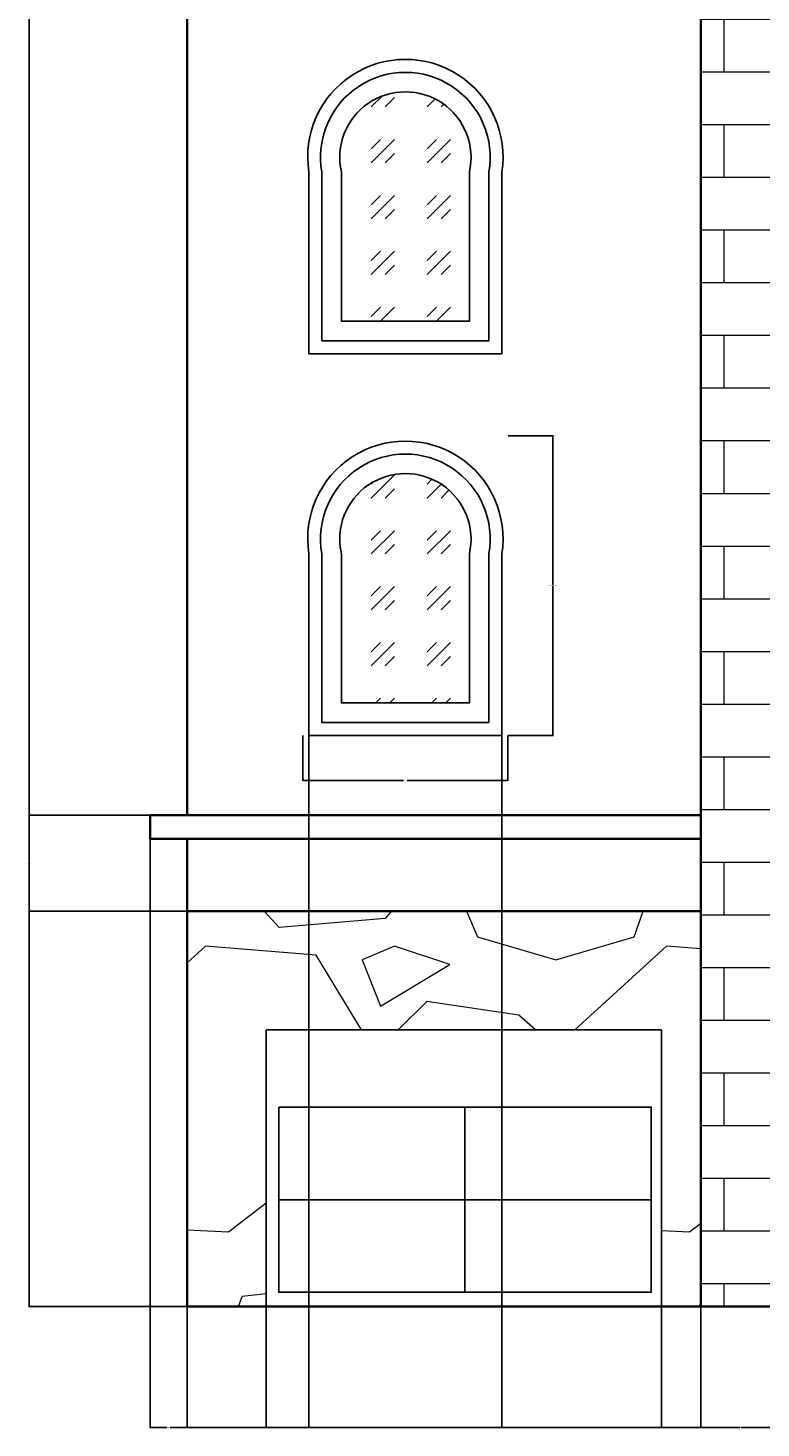
# Model space of a CAD drawing. Units: inches. Extents: x -19 to 556, y -28 to 766.
# Tile 1 of 3: x -19 to 203, y -28 to 397. Entities that reach past the tile are written whole.
import ezdxf

# ---------------------------------------------------------------- set-up
doc = ezdxf.new("R2010")
doc.units = ezdxf.units.IN
doc.header["$MEASUREMENT"] = 0
for name, color, linetype, lineweight in [('A-ANNO-DIMS', 2, 'Continuous', 18), ('A-DOOR', 3, 'Continuous', 25), ('A-ELEV', 7, 'Continuous', 35), ('A-GLAZ', 4, 'Continuous', 25), ('A-GLAZ-PATT', 252, 'Continuous', 13), ('A-WALL-PATT', 8, 'Continuous', 13)]:
    doc.layers.add(name, color=color, linetype=linetype, lineweight=lineweight)
doc.styles.get("Standard").update_dxf_attribs({"font": 'arial.ttf'})
doc.dimstyles.get("Standard").update_dxf_attribs({"dimtxt": 0.18, "dimasz": 0.18, "dimexe": 0.18, "dimexo": 0.0625, "dimgap": 0.09, "dimtad": 0, "dimtih": 1, "dimtoh": 1, "dimdec": 4, "dimzin": 0, "dimdsep": 46, "dimtxsty": 'Standard', "dimcen": 0.09, "dimadec": 0, "dimazin": 0, "dimtfac": 1, "dimtdec": 4, "dimtofl": 0, "dimtmove": 0, "dimatfit": 3, "dimfxl": 1, "dimtolj": 1, "dimtzin": 0, "dimarcsym": 0})

# ---------------------------------------------------------------- blocks, each defined once
blk = doc.blocks.new('WIN-ARCHED')
for points in [[(65.94, 237.64), (65.94, 182.48), (124.55, 182.48), (124.55, 237.64, 1.168317)], [(69.88, 237.64), (69.88, 186.43), (120.6, 186.43), (120.6, 237.64, 1.194508)], [(75.8, 237.64), (75.8, 192.35), (114.68, 192.35), (114.68, 237.64, 1.253731)]]:
    blk.add_lwpolyline(points, format="xyb", close=True)
blk = doc.blocks.new('DOOR-GARAGE')
for p, q in [((113.34, 69.59), (113.34, 13.35)), ((56.78, 41.47), (169.9, 41.47))]:
    blk.add_line(p, q)
blk.add_lwpolyline([(52.98, 9.07), (52.98, 93.07), (172.98, 93.07), (172.98, 9.07)])
blk.add_lwpolyline([(56.78, 69.59), (169.9, 69.59), (169.9, 13.35), (56.78, 13.35)], close=True)
blk = doc.blocks.new('*D4')
at = {"layer": 'A-ANNO-DIMS', "color": 0, "lineweight": -2, "transparency": 16777216}
for p, q in [((126.42, 273.47), (140.18, 273.47)), ((140, 273.29), (140, 228.16)), ((140, 182.66), (140, 227.79)), ((126.42, 182.48), (140.18, 182.48))]:
    blk.add_line(p, q, dxfattribs=at)
at = {"layer": 'A-ANNO-DIMS', "color": 0, "transparency": 16777216}
for points in [[(139.97, 273.29), (140.03, 273.29), (140, 273.47)], [(139.97, 182.66), (140.03, 182.66), (140, 182.48)]]:
    blk.add_solid(points, dxfattribs=at)
at = {"layer": 'Defpoints', "color": 0, "transparency": 16777216}
for p in [(126.35, 273.47), (140, 273.47), (126.35, 182.48)]:
    blk.add_point(p, dxfattribs=at)
at = {"layer": 'A-ANNO-DIMS', "color": 0, "transparency": 16777216, "insert": (140, 227.97), "char_height": 0.18, "attachment_point": 5}
blk.add_mtext('\\A1;ARCHED WINDOW 91 TYP.', dxfattribs=at)
blk = doc.blocks.new('*D5')
at = {"layer": 'A-ANNO-DIMS', "color": 0, "lineweight": -2, "transparency": 16777216}
for p, q in [((64.13, 182.42), (64.13, 168.66)), ((126.35, 182.42), (126.35, 168.66)), ((64.31, 168.84), (94.71, 168.84)), ((126.17, 168.84), (95.77, 168.84))]:
    blk.add_line(p, q, dxfattribs=at)
at = {"layer": 'A-ANNO-DIMS', "color": 0, "transparency": 16777216}
for points in [[(64.31, 168.87), (64.31, 168.81), (64.13, 168.84)], [(126.17, 168.87), (126.17, 168.81), (126.35, 168.84)]]:
    blk.add_solid(points, dxfattribs=at)
at = {"layer": 'Defpoints', "color": 0, "transparency": 16777216}
for p in [(64.13, 182.48), (126.35, 182.48), (126.35, 168.84)]:
    blk.add_point(p, dxfattribs=at)
at = {"layer": 'A-ANNO-DIMS', "color": 0, "transparency": 16777216, "insert": (95.24, 168.84), "char_height": 0.18, "attachment_point": 5}
blk.add_mtext('\\A1;62 TYP.', dxfattribs=at)
blk = doc.blocks.new('*D11')
at = {"layer": 'A-ANNO-DIMS', "color": 0, "lineweight": -2, "transparency": 16777216}
for p, q in [((174.92, 728.71), (-19.15, 728.71)), ((-18.97, 728.53), (-18.97, 369.07)), ((-18.97, 9.25), (-18.97, 368.71)), ((28.92, 9.07), (-19.15, 9.07))]:
    blk.add_line(p, q, dxfattribs=at)
at = {"layer": 'A-ANNO-DIMS', "color": 0, "transparency": 16777216}
for points in [[(-19, 728.53), (-18.94, 728.53), (-18.97, 728.71)], [(-19, 9.25), (-18.94, 9.25), (-18.97, 9.07)]]:
    blk.add_solid(points, dxfattribs=at)
at = {"layer": 'Defpoints', "color": 0, "transparency": 16777216}
for p in [(-18.97, 728.71), (174.98, 728.71), (28.98, 9.07)]:
    blk.add_point(p, dxfattribs=at)
at = {"layer": 'A-ANNO-DIMS', "color": 0, "transparency": 16777216, "insert": (-18.97, 368.89), "char_height": 0.18, "attachment_point": 5}
blk.add_mtext('\\A1;719.6', dxfattribs=at)
blk = doc.blocks.new('*D12')
at = {"layer": 'A-ANNO-DIMS', "color": 0, "lineweight": -2, "transparency": 16777216}
for p, q in [((28.92, 129.07), (-19.15, 129.07)), ((-18.97, 128.89), (-18.97, 69.26)), ((-18.97, 9.25), (-18.97, 68.89)), ((28.92, 9.07), (-19.15, 9.07))]:
    blk.add_line(p, q, dxfattribs=at)
at = {"layer": 'A-ANNO-DIMS', "color": 0, "transparency": 16777216}
for points in [[(-19, 128.89), (-18.94, 128.89), (-18.97, 129.07)], [(-19, 9.25), (-18.94, 9.25), (-18.97, 9.07)]]:
    blk.add_solid(points, dxfattribs=at)
at = {"layer": 'Defpoints', "color": 0, "transparency": 16777216}
for p in [(-18.97, 129.07), (28.98, 129.07), (28.98, 9.07)]:
    blk.add_point(p, dxfattribs=at)
at = {"layer": 'A-ANNO-DIMS', "color": 0, "transparency": 16777216, "insert": (-18.97, 69.07), "char_height": 0.18, "attachment_point": 5}
blk.add_mtext('\\A1;120', dxfattribs=at)
blk = doc.blocks.new('*D13')
at = {"layer": 'A-ANNO-DIMS', "color": 0, "lineweight": -2, "transparency": 16777216}
for p, q in [((17.71, 158.26), (-19.15, 158.26)), ((-18.97, 158.08), (-18.97, 143.85)), ((-18.97, 129.25), (-18.97, 143.49)), ((28.92, 129.07), (-19.15, 129.07))]:
    blk.add_line(p, q, dxfattribs=at)
at = {"layer": 'A-ANNO-DIMS', "color": 0, "transparency": 16777216}
for points in [[(-19, 158.08), (-18.94, 158.08), (-18.97, 158.26)], [(-19, 129.25), (-18.94, 129.25), (-18.97, 129.07)]]:
    blk.add_solid(points, dxfattribs=at)
at = {"layer": 'Defpoints', "color": 0, "transparency": 16777216}
for p in [(-18.97, 158.26), (17.78, 158.26), (28.98, 129.07)]:
    blk.add_point(p, dxfattribs=at)
at = {"layer": 'A-ANNO-DIMS', "color": 0, "transparency": 16777216, "insert": (-18.97, 143.67), "char_height": 0.18, "attachment_point": 5}
blk.add_mtext('\\A1;29.186', dxfattribs=at)
blk = doc.blocks.new('*D14')
at = {"layer": 'A-ANNO-DIMS', "color": 0, "lineweight": -2, "transparency": 16777216}
for p, q in [((28.92, 669.07), (-19.15, 669.07)), ((-18.97, 668.89), (-18.97, 413.85)), ((-18.97, 158.44), (-18.97, 413.49)), ((28.92, 158.26), (-19.15, 158.26))]:
    blk.add_line(p, q, dxfattribs=at)
at = {"layer": 'A-ANNO-DIMS', "color": 0, "transparency": 16777216}
for points in [[(-19, 668.89), (-18.94, 668.89), (-18.97, 669.07)], [(-19, 158.44), (-18.94, 158.44), (-18.97, 158.26)]]:
    blk.add_solid(points, dxfattribs=at)
at = {"layer": 'Defpoints', "color": 0, "transparency": 16777216}
for p in [(-18.97, 669.07), (28.98, 669.07), (28.98, 158.26)]:
    blk.add_point(p, dxfattribs=at)
at = {"layer": 'A-ANNO-DIMS', "color": 0, "transparency": 16777216, "insert": (-18.97, 413.67), "char_height": 0.18, "attachment_point": 5}
blk.add_mtext('\\A1;510.8', dxfattribs=at)
blk = doc.blocks.new('*D19')
at = {"layer": 'A-ANNO-DIMS', "color": 0, "lineweight": -2, "transparency": 16777216}
for p, q in [((52.98, 93.01), (52.98, -27.86)), ((172.98, 93.01), (172.98, -27.86)), ((53.16, -27.68), (112.7, -27.68)), ((172.8, -27.68), (113.26, -27.68))]:
    blk.add_line(p, q, dxfattribs=at)
at = {"layer": 'A-ANNO-DIMS', "color": 0, "transparency": 16777216}
for points in [[(53.16, -27.65), (53.16, -27.71), (52.98, -27.68)], [(172.8, -27.65), (172.8, -27.71), (172.98, -27.68)]]:
    blk.add_solid(points, dxfattribs=at)
at = {"layer": 'Defpoints', "color": 0, "transparency": 16777216}
for p in [(52.98, 93.07), (172.98, 93.07), (172.98, -27.68)]:
    blk.add_point(p, dxfattribs=at)
at = {"layer": 'A-ANNO-DIMS', "color": 0, "transparency": 16777216, "insert": (112.98, -27.68), "char_height": 0.18, "attachment_point": 5}
blk.add_mtext('\\A1;120', dxfattribs=at)
blk = doc.blocks.new('*D20')
at = {"layer": 'A-ANNO-DIMS', "color": 0, "lineweight": -2, "transparency": 16777216}
for p, q in [((28.98, 9.01), (28.98, -27.86)), ((52.98, 9.01), (52.98, -27.86)), ((29.16, -27.68), (40.76, -27.68)), ((52.8, -27.68), (41.2, -27.68))]:
    blk.add_line(p, q, dxfattribs=at)
at = {"layer": 'A-ANNO-DIMS', "color": 0, "transparency": 16777216}
for points in [[(29.16, -27.65), (29.16, -27.71), (28.98, -27.68)], [(52.8, -27.65), (52.8, -27.71), (52.98, -27.68)]]:
    blk.add_solid(points, dxfattribs=at)
at = {"layer": 'Defpoints', "color": 0, "transparency": 16777216}
for p in [(28.98, 9.07), (52.98, 9.07), (52.98, -27.68)]:
    blk.add_point(p, dxfattribs=at)
at = {"layer": 'A-ANNO-DIMS', "color": 0, "transparency": 16777216, "insert": (40.98, -27.68), "char_height": 0.18, "attachment_point": 5}
blk.add_mtext('\\A1;24', dxfattribs=at)
blk = doc.blocks.new('*D29')
at = {"layer": 'A-ANNO-DIMS', "color": 0, "lineweight": -2, "transparency": 16777216}
for p, q in [((17.78, 150.98), (17.78, -27.86)), ((28.98, 9.01), (28.98, -27.86)), ((17.96, -27.68), (22.93, -27.68)), ((28.8, -27.68), (23.84, -27.68))]:
    blk.add_line(p, q, dxfattribs=at)
at = {"layer": 'A-ANNO-DIMS', "color": 0, "transparency": 16777216}
for points in [[(17.96, -27.65), (17.96, -27.71), (17.78, -27.68)], [(28.8, -27.65), (28.8, -27.71), (28.98, -27.68)]]:
    blk.add_solid(points, dxfattribs=at)
at = {"layer": 'Defpoints', "color": 0, "transparency": 16777216}
for p in [(17.78, 151.04), (28.98, 9.07), (28.98, -27.68)]:
    blk.add_point(p, dxfattribs=at)
at = {"layer": 'A-ANNO-DIMS', "color": 0, "transparency": 16777216, "insert": (23.38, -27.68), "char_height": 0.18, "attachment_point": 5}
blk.add_mtext('\\A1;11.206', dxfattribs=at)
blk = doc.blocks.new('*D30')
at = {"layer": 'A-ANNO-DIMS', "color": 0, "lineweight": -2, "transparency": 16777216}
for p, q in [((65.94, 182.42), (65.94, -27.86)), ((28.98, 9.01), (28.98, -27.86)), ((29.16, -27.68), (47.07, -27.68)), ((65.76, -27.68), (47.85, -27.68))]:
    blk.add_line(p, q, dxfattribs=at)
at = {"layer": 'A-ANNO-DIMS', "color": 0, "transparency": 16777216}
for points in [[(29.16, -27.65), (29.16, -27.71), (28.98, -27.68)], [(65.76, -27.65), (65.76, -27.71), (65.94, -27.68)]]:
    blk.add_solid(points, dxfattribs=at)
at = {"layer": 'Defpoints', "color": 0, "transparency": 16777216}
for p in [(65.94, 182.48), (28.98, 9.07), (65.94, -27.68)]:
    blk.add_point(p, dxfattribs=at)
at = {"layer": 'A-ANNO-DIMS', "color": 0, "transparency": 16777216, "insert": (47.46, -27.68), "char_height": 0.18, "attachment_point": 5}
blk.add_mtext('\\A1;36.95', dxfattribs=at)
blk = doc.blocks.new('*D31')
at = {"layer": 'A-ANNO-DIMS', "color": 0, "lineweight": -2, "transparency": 16777216}
for p, q in [((65.94, 182.42), (65.94, -27.86)), ((124.55, 182.42), (124.55, -27.86)), ((66.12, -27.68), (94.87, -27.68)), ((124.37, -27.68), (95.62, -27.68))]:
    blk.add_line(p, q, dxfattribs=at)
at = {"layer": 'A-ANNO-DIMS', "color": 0, "transparency": 16777216}
for points in [[(66.12, -27.65), (66.12, -27.71), (65.94, -27.68)], [(124.37, -27.65), (124.37, -27.71), (124.55, -27.68)]]:
    blk.add_solid(points, dxfattribs=at)
at = {"layer": 'Defpoints', "color": 0, "transparency": 16777216}
for p in [(65.94, 182.48), (124.55, 182.48), (124.55, -27.68)]:
    blk.add_point(p, dxfattribs=at)
at = {"layer": 'A-ANNO-DIMS', "color": 0, "transparency": 16777216, "insert": (95.24, -27.68), "char_height": 0.18, "attachment_point": 5}
blk.add_mtext('\\A1;58.61', dxfattribs=at)
blk = doc.blocks.new('*D32')
at = {"layer": 'A-ANNO-DIMS', "color": 0, "lineweight": -2, "transparency": 16777216}
for p, q in [((124.55, 182.42), (124.55, -27.86)), ((184.98, 9.01), (184.98, -27.86)), ((124.73, -27.68), (154.37, -27.68)), ((184.8, -27.68), (155.16, -27.68))]:
    blk.add_line(p, q, dxfattribs=at)
at = {"layer": 'A-ANNO-DIMS', "color": 0, "transparency": 16777216}
for points in [[(124.73, -27.65), (124.73, -27.71), (124.55, -27.68)], [(184.8, -27.65), (184.8, -27.71), (184.98, -27.68)]]:
    blk.add_solid(points, dxfattribs=at)
at = {"layer": 'Defpoints', "color": 0, "transparency": 16777216}
for p in [(124.55, 182.48), (184.98, 9.07), (184.98, -27.68)]:
    blk.add_point(p, dxfattribs=at)
at = {"layer": 'A-ANNO-DIMS', "color": 0, "transparency": 16777216, "insert": (154.77, -27.68), "char_height": 0.18, "attachment_point": 5}
blk.add_mtext('\\A1;60.43', dxfattribs=at)
blk = doc.blocks.new('*D33')
at = {"layer": 'A-ANNO-DIMS', "color": 0, "lineweight": -2, "transparency": 16777216}
for p, q in [((184.98, 9.01), (184.98, -27.86)), ((208.98, 9.01), (208.98, -27.86)), ((185.16, -27.68), (196.76, -27.68)), ((208.8, -27.68), (197.2, -27.68))]:
    blk.add_line(p, q, dxfattribs=at)
at = {"layer": 'A-ANNO-DIMS', "color": 0, "transparency": 16777216}
for points in [[(185.16, -27.65), (185.16, -27.71), (184.98, -27.68)], [(208.8, -27.65), (208.8, -27.71), (208.98, -27.68)]]:
    blk.add_solid(points, dxfattribs=at)
at = {"layer": 'Defpoints', "color": 0, "transparency": 16777216}
for p in [(184.98, 9.07), (208.98, 9.07), (208.98, -27.68)]:
    blk.add_point(p, dxfattribs=at)
at = {"layer": 'A-ANNO-DIMS', "color": 0, "transparency": 16777216, "insert": (196.98, -27.68), "char_height": 0.18, "attachment_point": 5}
blk.add_mtext('\\A1;24', dxfattribs=at)

msp = doc.modelspace()

# ---------------------------------------------------------------- hatches: boundary and pattern name
at = {"layer": 'A-GLAZ-PATT'}
h = msp.add_hatch(dxfattribs=at)
h.set_pattern_fill('GOST_GLASS', color=256, scale=2)
h.set_pattern_definition([(45, (0, 0), (16.97056, 0), [10, -14]), (45, (4.243, 0), (16.97056, 0), [4, -20]), (45, (0, 4.243), (16.97056, 0), [4, -20])])
h.paths.add_polyline_path([(114.6834, 591.8123, 1.25373075), (75.801, 591.8123), (75.801, 546.5249), (114.6834, 546.5249)])
h.paths.add_polyline_path([(454.2051, 591.8123, 1.25373075), (415.3227, 591.8123), (415.3227, 546.5249), (454.2051, 546.5249)])
h.paths.add_polyline_path([(288.5244, 564.1792, 1.25373075), (249.6421, 564.1792), (249.6421, 518.8919), (288.5244, 518.8919)])
h.paths.add_polyline_path([(114.6834, 469.356, 1.25373075), (75.801, 469.356), (75.801, 424.0687), (114.6834, 424.0687)])
h.paths.add_polyline_path([(288.5244, 420.4043, 1.25373075), (249.6421, 420.4043), (249.6421, 375.1169), (288.5244, 375.1169)])
h.paths.add_polyline_path([(454.2051, 469.356, 1.25373075), (415.3227, 469.356), (415.3227, 424.0687), (454.2051, 424.0687)])
h.paths.add_polyline_path([(454.2051, 353.5792, 1.25373075), (415.3227, 353.5792), (415.3227, 308.2919), (454.2051, 308.2919)])
h.paths.add_polyline_path([(454.2051, 237.6357, 1.25373075), (415.3227, 237.6357), (415.3227, 192.3483), (454.2051, 192.3483)])
h.paths.add_polyline_path([(288.5244, 280.5161, 1.25373075), (249.6421, 280.5161), (249.6421, 235.2288), (288.5244, 235.2288)])
h.paths.add_polyline_path([(114.6834, 237.6357, 1.25373075), (75.801, 237.6357), (75.801, 192.3483), (114.6834, 192.3483)])
h.paths.add_polyline_path([(114.6834, 353.5792, 1.25373075), (75.801, 353.5792), (75.801, 308.2919), (114.6834, 308.2919)])
at = {"layer": 'A-WALL-PATT'}
h = msp.add_hatch(dxfattribs=at)
h.set_pattern_fill('AR-B816', color=256, scale=2)
h.paths.add_polyline_path([(208.9833, 669.0741), (184.9833, 669.0741), (184.9833, 129.0741), (184.9833, 9.0741), (208.9833, 9.0741), (208.9833, 129.0741)])
h.paths.add_polyline_path([(352.9833, 669.0741), (328.9833, 669.0741), (328.9833, 129.0741), (328.9833, 9.0741), (352.9833, 9.0741), (352.9833, 129.0741)])
h = msp.add_hatch(dxfattribs=at)
h.set_pattern_fill('GRAVEL', color=256, scale=140)
h.paths.add_polyline_path([(184.9833, 129.0741), (28.9833, 129.0741), (28.9833, 9.0741), (52.9833, 9.0741), (52.9833, 93.0741), (172.9833, 93.0741), (172.9833, 9.0741), (184.9833, 9.0741)])
h.paths.add_polyline_path([(508.9833, 129.0741), (352.9833, 129.0741), (352.9833, 9.0741), (364.9833, 9.0741), (364.9833, 93.0741), (484.9833, 93.0741), (484.9833, 9.0741), (508.9833, 9.0741)])

# ---------------------------------------------------------------- linework, layer by layer
at = {"layer": 'A-ELEV'}
for p, q in [((184.9833, 669.0741), (184.9833, 129.0741)), ((28.9833, 158.26), (17.7774, 158.26)), ((17.7774, 158.26), (17.7774, 151.0378)), ((17.7774, 151.0378), (184.9833, 151.0378))]:
    msp.add_line(p, q, dxfattribs=at)
for points in [[(507.6136, 158.26), (507.6136, 669.0741), (28.9833, 669.0741), (28.9833, 158.26)], [(184.9833, 158.26), (28.9833, 158.26)], [(28.9833, 151.0378), (28.9833, 129.0741), (184.9833, 129.0741)], [(28.9833, 151.0378), (28.9833, 129.0741), (184.9833, 129.0741), (184.9833, 9.0741)], [(184.9833, 129.0741), (28.9833, 129.0741), (28.9833, 9.0741), (508.9833, 9.0741), (508.9833, 129.0741), (352.9833, 129.0741)]]:
    msp.add_lwpolyline(points, dxfattribs=at)

# ---------------------------------------------------------------- block references
at = {"layer": 'A-DOOR'}
msp.add_blockref('DOOR-GARAGE', (0, 0), dxfattribs=at)
at = {"layer": 'A-GLAZ'}
for p in [(0, 115.9436), (0, 0)]:
    msp.add_blockref('WIN-ARCHED', p, dxfattribs=at)

# ---------------------------------------------------------------- dimensions: what is measured, and where the dimension line sits
at = {"layer": 'A-ANNO-DIMS'}
for base, p1, p2, override, picture, middle in [((-18.9726, 728.7105), (28.9833, 9.0741), (174.98, 728.7105), {"dimdec": 1, "dimlfac": 1, "dimrnd": 0, "dimzin": 0, "dimdsep": 46, "dimlunit": 2}, '*D11', (-18.9726, 368.8923)), ((-18.9726, 669.0741), (28.9833, 158.26), (28.9833, 669.0741), {"dimdec": 1, "dimlfac": 1, "dimrnd": 0, "dimzin": 0, "dimdsep": 46, "dimlunit": 2}, '*D14', (-18.9726, 413.6671)), ((-18.9726, 158.26), (28.9833, 129.0741), (17.7774, 158.26), {"dimdec": 3, "dimlfac": 1, "dimrnd": 0, "dimzin": 0, "dimdsep": 46, "dimlunit": 2}, '*D13', (-18.9726, 143.6671)), ((-18.9726, 129.0741), (28.9833, 9.0741), (28.9833, 129.0741), {"dimdec": 0, "dimlfac": 1, "dimrnd": 0, "dimzin": 0, "dimdsep": 46, "dimlunit": 2}, '*D12', (-18.9726, 69.0741))]:
    dim = msp.add_linear_dim(base=base, p1=p1, p2=p2, angle=90, dimstyle='Standard', override=override, dxfattribs=at)
    dim.commit()
    dim.dimension.update_dxf_attribs({"geometry": picture, "text_midpoint": middle})
dim = msp.add_linear_dim(base=(140.0022, 273.4666), p1=(126.3546, 182.4827), p2=(126.3546, 273.4666), angle=90, text='ARCHED WINDOW <> TYP.', dimstyle='Standard', override={"dimdec": 0, "dimlfac": 1, "dimrnd": 0, "dimzin": 0, "dimdsep": 46, "dimlunit": 2}, dxfattribs=at)
dim.commit()
dim.dimension.update_dxf_attribs({"geometry": '*D4', "text_midpoint": (140.0022, 227.9746)})
for base, p1, p2, override, picture, middle in [((65.9354, -27.6759), (28.9833, 9.0741), (65.9354, 182.4827), {"dimdec": 2, "dimlfac": 1, "dimrnd": 0, "dimzin": 0, "dimdsep": 46, "dimlunit": 2}, '*D30', (47.4593, -27.6759)), ((124.549, -27.6759), (65.9354, 182.4827), (124.549, 182.4827), {"dimdec": 2, "dimlfac": 1, "dimrnd": 0, "dimzin": 0, "dimdsep": 46, "dimlunit": 2}, '*D31', (95.2422, -27.6759)), ((184.9833, -27.6759), (124.549, 182.4827), (184.9833, 9.0741), {"dimdec": 2, "dimlfac": 1, "dimrnd": 0, "dimzin": 0, "dimdsep": 46, "dimlunit": 2}, '*D32', (154.7662, -27.6759)), ((28.9833, -27.6759), (17.7774, 151.0378), (28.9833, 9.0741), {"dimdec": 3, "dimlfac": 1, "dimrnd": 0, "dimzin": 0, "dimdsep": 46, "dimlunit": 2}, '*D29', (23.3804, -27.6759)), ((172.9833, -27.6759), (52.9833, 93.0741), (172.9833, 93.0741), {"dimdec": 0, "dimlfac": 1, "dimrnd": 0, "dimzin": 0, "dimdsep": 46, "dimlunit": 2}, '*D19', (112.9833, -27.6759)), ((52.9833, -27.6759), (28.9833, 9.0741), (52.9833, 9.0741), {"dimdec": 0, "dimlfac": 1, "dimrnd": 0, "dimzin": 0, "dimdsep": 46, "dimlunit": 2}, '*D20', (40.9833, -27.6759)), ((208.9833, -27.6759), (184.9833, 9.0741), (208.9833, 9.0741), {"dimdec": 0, "dimlfac": 1, "dimrnd": 0, "dimzin": 0, "dimdsep": 46, "dimlunit": 2}, '*D33', (196.9833, -27.6759))]:
    dim = msp.add_linear_dim(base=base, p1=p1, p2=p2, dimstyle='Standard', override=override, dxfattribs=at)
    dim.commit()
    dim.dimension.update_dxf_attribs({"geometry": picture, "text_midpoint": middle})
dim = msp.add_linear_dim(base=(126.3546, 168.8351), p1=(64.1298, 182.4827), p2=(126.3546, 182.4827), text='<> TYP.', dimstyle='Standard', override={"dimdec": 0, "dimlfac": 1, "dimrnd": 0, "dimzin": 0, "dimdsep": 46, "dimlunit": 2}, dxfattribs=at)
dim.commit()
dim.dimension.update_dxf_attribs({"geometry": '*D5', "text_midpoint": (95.2422, 168.8351)})

doc.saveas('drawing.dxf')
